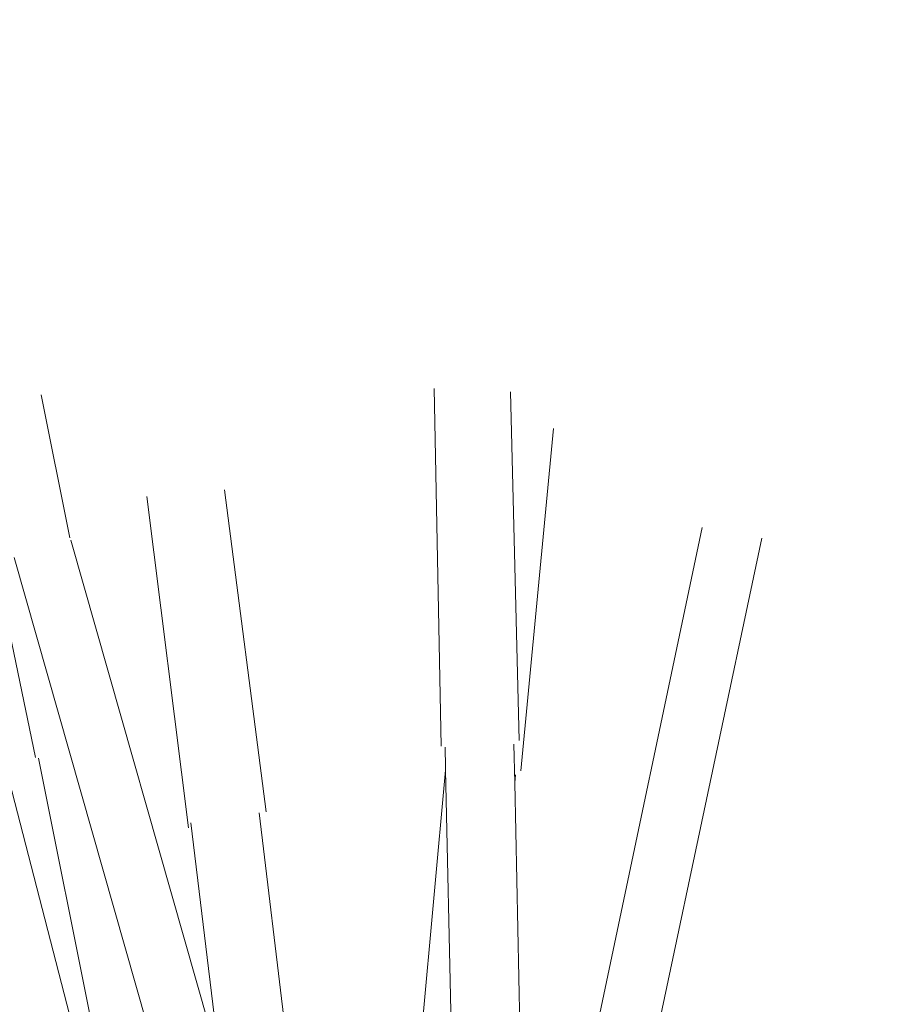
# Model space of a CAD drawing. Units: millimetres. Extents: x 7894 to 8038, y 6851 to 6951.
# Tile 35 of 49: x 7965.741 to 7968.188, y 6925.713 to 6928.453. Entities that reach past the tile are written whole.
import ezdxf

# ---------------------------------------------------------------- set-up
doc = ezdxf.new("R2010")
doc.units = ezdxf.units.MM
doc.layers.add('A-ANNO-DIMS', color=2, linetype='Continuous', lineweight=18)
doc.layers.add('A-FURN-ACCS', color=8, linetype='Continuous', lineweight=13)
doc.styles.get("Standard").update_dxf_attribs({"font": 'arial.ttf'})
doc.dimstyles.new('ISO-25', dxfattribs={"dimtxt": 1, "dimasz": 1, "dimexe": 1.25, "dimexo": 0.625, "dimtad": 1, "dimdec": 0, "dimlunit": 4, "dimtxsty": 'Standard', "dimcen": 2.5, "dimclrt": 1, "dimadec": 0, "dimazin": 0, "dimtfac": 1, "dimtdec": 0, "dimtmove": 0, "dimatfit": 3, "dimfxl": 1, "dimarcsym": 0})

# ---------------------------------------------------------------- blocks, each defined once
blk = doc.blocks.new('DISPLAY-REED-SPRAY')
for p, q in [((1.5483, 0.9938), (1.529, 1.9891)), ((1.7657, 1.0095), (1.7415, 1.9798)), ((0.5154, 1.5733), (0.4354, 1.9715)), ((0.2181, 1.9336), (0.4198, 0.9626)), ((1.7698, 0.9258), (1.8607, 1.8783)), ((1.0617, 0.8114), (0.9453, 1.7069)), ((0.8459, 0.7666), (0.7293, 1.6887)), ((0.5782, 0.0032), (0.1619, 1.6106)), ((1.9375, 0.0029), (2.2747, 1.6026)), ((0, 1.5725), (0.4056, 0.0011)), ((0.9346, 0.1034), (0.5185, 1.5674)), ((2.1079, 0.0011), (2.44, 1.5729)), ((0.7924, 0), (0.3606, 1.5186)), ((1.5597, 0.991), (1.5609, 0.9349)), ((1.753, 0.8924), (1.7508, 0.9993)), ((0.6196, 0.0033), (0.4281, 0.9603)), ((1.5603, 0.9272), (1.5609, 0.9349)), ((1.4766, 0.0028), (1.5603, 0.9272)), ((1.5603, 0.9272), (1.5804, 0.0032)), ((1.753, 0.8924), (1.7551, 0.9145)), ((1.7713, 0.0032), (1.753, 0.8924)), ((1.1386, 0.003), (1.042, 0.8085)), ((0.9346, 0.1034), (0.8517, 0.7803)), ((0.9634, 0.002), (0.9346, 0.1034))]:
    blk.add_line(p, q)
blk = doc.blocks.new('*D23')
at = {"layer": 'A-ANNO-DIMS', "color": 0, "lineweight": -2, "transparency": 16777216}
for p, q in [((7940.0888, 6907.098), (7940.0888, 6947.7928)), ((7971.9356, 6928.989), (7971.9356, 6947.7928)), ((7941.0888, 6946.5428), (7970.9356, 6946.5428))]:
    blk.add_line(p, q, dxfattribs=at)
at = {"layer": 'A-ANNO-DIMS', "color": 0, "transparency": 16777216}
for points in [[(7941.0888, 6946.7095), (7941.0888, 6946.3762), (7940.0888, 6946.5428)], [(7970.9356, 6946.7095), (7970.9356, 6946.3762), (7971.9356, 6946.5428)]]:
    blk.add_solid(points, dxfattribs=at)
at = {"layer": 'Defpoints', "color": 0, "transparency": 16777216}
for p in [(7971.9356, 6946.5428), (7971.9356, 6928.364), (7940.0888, 6906.473)]:
    blk.add_point(p, dxfattribs=at)
at = {"layer": 'A-ANNO-DIMS', "color": 1, "transparency": 16777216, "insert": (7956.0122, 6947.6784), "char_height": 1, "attachment_point": 5}
blk.add_mtext('2\'-8"', dxfattribs=at)
blk = doc.blocks.new('*D28')
at = {"layer": 'A-ANNO-DIMS', "color": 0, "lineweight": -2, "transparency": 16777216}
for p, q in [((7960.8854, 6936.8804), (7975.2272, 6936.8804)), ((7973.9772, 6935.8804), (7973.9772, 6923.6283)), ((7971.8421, 6922.6283), (7975.2272, 6922.6283))]:
    blk.add_line(p, q, dxfattribs=at)
at = {"layer": 'A-ANNO-DIMS', "color": 0, "transparency": 16777216}
for points in [[(7973.8105, 6935.8804), (7974.1439, 6935.8804), (7973.9772, 6936.8804)], [(7973.8105, 6923.6283), (7974.1439, 6923.6283), (7973.9772, 6922.6283)]]:
    blk.add_solid(points, dxfattribs=at)
at = {"layer": 'Defpoints', "color": 0, "transparency": 16777216}
for p in [(7960.2604, 6936.8804), (7971.2171, 6922.6283), (7973.9772, 6922.6283)]:
    blk.add_point(p, dxfattribs=at)
at = {"layer": 'A-ANNO-DIMS', "color": 1, "transparency": 16777216, "insert": (7972.8351, 6929.7543), "char_height": 1, "attachment_point": 5, "rotation": 90}
blk.add_mtext('1\'-2 1/2"', dxfattribs=at)
blk = doc.blocks.new('*D31')
at = {"layer": 'A-ANNO-DIMS', "color": 0, "lineweight": -2, "transparency": 16777216}
for p, q in [((7973.9772, 6921.7198), (7973.9772, 6926.628)), ((7949.8107, 6920.7198), (7975.2272, 6920.7198)), ((7973.9772, 6918.7198), (7973.9772, 6920.7198)), ((7950.9654, 6918.7198), (7975.2272, 6918.7198)), ((7973.9772, 6917.7198), (7973.9772, 6916.7198))]:
    blk.add_line(p, q, dxfattribs=at)
at = {"layer": 'A-ANNO-DIMS', "color": 0, "transparency": 16777216}
for points in [[(7973.8105, 6921.7198), (7974.1439, 6921.7198), (7973.9772, 6920.7198)], [(7973.8105, 6917.7198), (7974.1439, 6917.7198), (7973.9772, 6918.7198)]]:
    blk.add_solid(points, dxfattribs=at)
at = {"layer": 'Defpoints', "color": 0, "transparency": 16777216}
for p in [(7949.1857, 6920.7198), (7973.9772, 6920.7198), (7950.3404, 6918.7198)]:
    blk.add_point(p, dxfattribs=at)
at = {"layer": 'A-ANNO-DIMS', "color": 1, "transparency": 16777216, "insert": (7972.8416, 6924.6739), "char_height": 1, "attachment_point": 5, "rotation": 90}
blk.add_mtext('0\'-2"', dxfattribs=at)

msp = doc.modelspace()

# ---------------------------------------------------------------- block references
at = {"layer": 'A-FURN-ACCS'}
msp.add_blockref('DISPLAY-REED-SPRAY', (7965.365, 6925.4377), dxfattribs=at)

# ---------------------------------------------------------------- dimensions: what is measured, and where the dimension line sits
at = {"layer": 'A-ANNO-DIMS'}
dim = msp.add_linear_dim(base=(7971.9356, 6946.5428), p1=(7940.0888, 6906.473), p2=(7971.9356, 6928.364), dimstyle='ISO-25', override={"dimdec": 1, "dimlfac": 1, "dimrnd": 0, "dimzin": 1, "dimdsep": 46, "dimlunit": 4, "dimfrac": 2}, dxfattribs=at)
dim.commit()
dim.dimension.update_dxf_attribs({"geometry": '*D23', "text_midpoint": (7956.0122, 6947.6784)})
for base, p1, p2, picture, middle in [((7973.9772, 6922.6283), (7960.2604, 6936.8804), (7971.2171, 6922.6283), '*D28', (7972.8351, 6929.7543)), ((7973.9772, 6920.7198), (7950.3404, 6918.7198), (7949.1857, 6920.7198), '*D31', (7972.8416, 6924.6739))]:
    dim = msp.add_linear_dim(base=base, p1=p1, p2=p2, angle=90, dimstyle='ISO-25', override={"dimdec": 1, "dimlfac": 1, "dimrnd": 0, "dimzin": 1, "dimdsep": 46, "dimlunit": 4, "dimfrac": 2}, dxfattribs=at)
    dim.commit()
    dim.dimension.update_dxf_attribs({"geometry": picture, "text_midpoint": middle})

doc.saveas('drawing.dxf')
